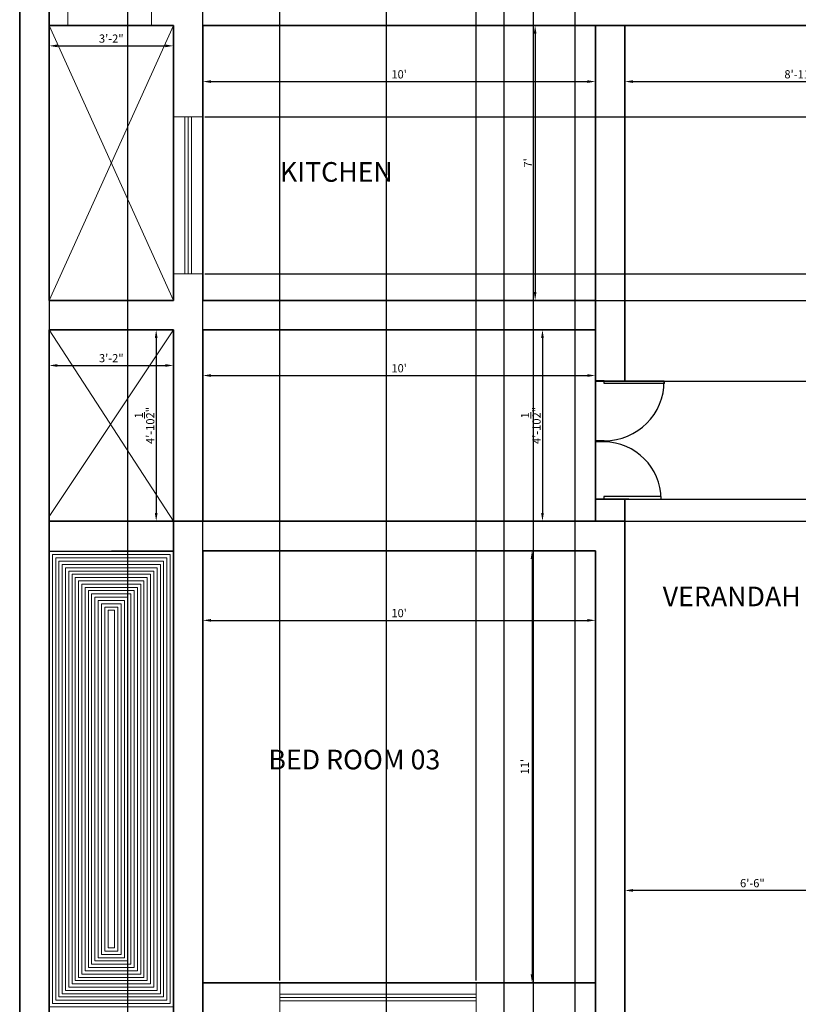
# Model space of a CAD drawing. Units: inches. Extents: x 2178 to 2667, y 1439 to 2239.
# Tile 2 of 5: x 2218 to 2456, y 1590 to 1891. Entities that reach past the tile are written whole.
import ezdxf

# ---------------------------------------------------------------- set-up
doc = ezdxf.new("R2010")
doc.units = ezdxf.units.IN
for name, color, linetype, lineweight in [('A-ANNO-DIMS', 2, 'Continuous', 18), ('A-AREA-IDEN', 7, 'Continuous', 18), ('A-DOOR', 3, 'Continuous', 25), ('A-FLOR-OPEN', 8, 'Continuous', 18), ('A-FLOR-PATT', 252, 'Continuous', 13), ('A-GLAZ', 4, 'Continuous', 18), ('A-WALL', 7, 'Continuous', 35)]:
    doc.layers.add(name, color=color, linetype=linetype, lineweight=lineweight)
doc.styles.get("Standard").update_dxf_attribs({"font": 'arial.ttf'})
doc.dimstyles.new('Copy of ISO-25', dxfattribs={"dimtxt": 2.5, "dimasz": 2.5, "dimexe": 1.25, "dimexo": 0.625, "dimtad": 1, "dimdec": 1, "dimlunit": 4, "dimtxsty": 'Standard', "dimcen": 2.5, "dimadec": 0, "dimazin": 0, "dimtfac": 1, "dimtdec": 1, "dimtmove": 0, "dimatfit": 3, "dimfxl": 1, "dimarcsym": 0})

# ---------------------------------------------------------------- blocks, each defined once
blk = doc.blocks.new('*D11')
at = {"layer": 'A-ANNO-DIMS', "color": 0, "lineweight": -2, "transparency": 16777216}
for p, q in [((2273.53, 1888.41), (2273.53, 1870.62)), ((2393.53, 1888.41), (2393.53, 1870.62)), ((2276.03, 1871.87), (2391.03, 1871.87))]:
    blk.add_line(p, q, dxfattribs=at)
at = {"layer": 'A-ANNO-DIMS', "color": 0, "transparency": 16777216}
for points in [[(2276.03, 1872.29), (2276.03, 1871.45), (2273.53, 1871.87)], [(2391.03, 1872.29), (2391.03, 1871.45), (2393.53, 1871.87)]]:
    blk.add_solid(points, dxfattribs=at)
at = {"layer": 'Defpoints', "color": 0, "transparency": 16777216}
for p in [(2273.53, 1889.03), (2393.53, 1889.03), (2393.53, 1871.87)]:
    blk.add_point(p, dxfattribs=at)
at = {"layer": 'A-ANNO-DIMS', "color": 0, "transparency": 16777216, "insert": (2333.53, 1873.77), "char_height": 2.5, "attachment_point": 5}
blk.add_mtext("10'", dxfattribs=at)
blk = doc.blocks.new('*D12')
at = {"layer": 'A-ANNO-DIMS', "color": 0, "lineweight": -2, "transparency": 16777216}
for p, q in [((2392.9, 1889.03), (2373.87, 1889.03)), ((2375.12, 1886.53), (2375.12, 1807.53)), ((2392.9, 1805.03), (2373.87, 1805.03))]:
    blk.add_line(p, q, dxfattribs=at)
at = {"layer": 'A-ANNO-DIMS', "color": 0, "transparency": 16777216}
for points in [[(2374.7, 1886.53), (2375.53, 1886.53), (2375.12, 1889.03)], [(2374.7, 1807.53), (2375.53, 1807.53), (2375.12, 1805.03)]]:
    blk.add_solid(points, dxfattribs=at)
at = {"layer": 'Defpoints', "color": 0, "transparency": 16777216}
for p in [(2393.53, 1889.03), (2375.12, 1805.03), (2393.53, 1805.03)]:
    blk.add_point(p, dxfattribs=at)
at = {"layer": 'A-ANNO-DIMS', "color": 0, "transparency": 16777216, "insert": (2373.24, 1847.03), "char_height": 2.5, "attachment_point": 5, "rotation": 90}
blk.add_mtext("7'", dxfattribs=at)
blk = doc.blocks.new('*D13')
at = {"layer": 'A-ANNO-DIMS', "color": 0, "lineweight": -2, "transparency": 16777216}
for p, q in [((2226.53, 1888.41), (2226.53, 1881.54)), ((2264.53, 1888.41), (2264.53, 1881.54)), ((2229.03, 1882.79), (2262.03, 1882.79))]:
    blk.add_line(p, q, dxfattribs=at)
at = {"layer": 'A-ANNO-DIMS', "color": 0, "transparency": 16777216}
for points in [[(2229.03, 1883.2), (2229.03, 1882.37), (2226.53, 1882.79)], [(2262.03, 1883.2), (2262.03, 1882.37), (2264.53, 1882.79)]]:
    blk.add_solid(points, dxfattribs=at)
at = {"layer": 'Defpoints', "color": 0, "transparency": 16777216}
for p in [(2226.53, 1889.03), (2264.53, 1889.03), (2264.53, 1882.79)]:
    blk.add_point(p, dxfattribs=at)
at = {"layer": 'A-ANNO-DIMS', "color": 0, "transparency": 16777216, "insert": (2245.53, 1884.69), "char_height": 2.5, "attachment_point": 5}
blk.add_mtext('3\'-2"', dxfattribs=at)
blk = doc.blocks.new('*D14')
at = {"layer": 'A-ANNO-DIMS', "color": 0, "lineweight": -2, "transparency": 16777216}
for p, q in [((2402.53, 1888.41), (2402.53, 1870.62)), ((2509.53, 1888.41), (2509.53, 1870.62)), ((2405.03, 1871.87), (2507.03, 1871.87))]:
    blk.add_line(p, q, dxfattribs=at)
at = {"layer": 'A-ANNO-DIMS', "color": 0, "transparency": 16777216}
for points in [[(2405.03, 1872.29), (2405.03, 1871.45), (2402.53, 1871.87)], [(2507.03, 1872.29), (2507.03, 1871.45), (2509.53, 1871.87)]]:
    blk.add_solid(points, dxfattribs=at)
at = {"layer": 'Defpoints', "color": 0, "transparency": 16777216}
for p in [(2402.53, 1889.03), (2509.53, 1889.03), (2509.53, 1871.87)]:
    blk.add_point(p, dxfattribs=at)
at = {"layer": 'A-ANNO-DIMS', "color": 0, "transparency": 16777216, "insert": (2456.03, 1873.77), "char_height": 2.5, "attachment_point": 5}
blk.add_mtext('8\'-11"', dxfattribs=at)
blk = doc.blocks.new('*D15')
at = {"layer": 'A-ANNO-DIMS', "color": 0, "lineweight": -2, "transparency": 16777216}
for p, q in [((2392.9, 1796.03), (2376.11, 1796.03)), ((2377.36, 1793.53), (2377.36, 1740.03)), ((2392.9, 1737.53), (2376.11, 1737.53))]:
    blk.add_line(p, q, dxfattribs=at)
at = {"layer": 'A-ANNO-DIMS', "color": 0, "transparency": 16777216}
for points in [[(2376.95, 1793.53), (2377.78, 1793.53), (2377.36, 1796.03)], [(2376.95, 1740.03), (2377.78, 1740.03), (2377.36, 1737.53)]]:
    blk.add_solid(points, dxfattribs=at)
at = {"layer": 'Defpoints', "color": 0, "transparency": 16777216}
for p in [(2393.53, 1796.03), (2377.36, 1737.53), (2393.53, 1737.53)]:
    blk.add_point(p, dxfattribs=at)
at = {"layer": 'A-ANNO-DIMS', "color": 0, "transparency": 16777216, "insert": (2373.79, 1766.78), "char_height": 2.5, "attachment_point": 5, "rotation": 90}
blk.add_mtext('4\'-10{\\H1x;\\S1/2;}"', dxfattribs=at)
blk = doc.blocks.new('*D16')
at = {"layer": 'A-ANNO-DIMS', "color": 0, "lineweight": -2, "transparency": 16777216}
for p, q in [((2226.53, 1795.41), (2226.53, 1783.88)), ((2264.53, 1795.41), (2264.53, 1783.88)), ((2229.03, 1785.13), (2262.03, 1785.13))]:
    blk.add_line(p, q, dxfattribs=at)
at = {"layer": 'A-ANNO-DIMS', "color": 0, "transparency": 16777216}
for points in [[(2229.03, 1785.54), (2229.03, 1784.71), (2226.53, 1785.13)], [(2262.03, 1785.54), (2262.03, 1784.71), (2264.53, 1785.13)]]:
    blk.add_solid(points, dxfattribs=at)
at = {"layer": 'Defpoints', "color": 0, "transparency": 16777216}
for p in [(2226.53, 1796.03), (2264.53, 1796.03), (2264.53, 1785.13)]:
    blk.add_point(p, dxfattribs=at)
at = {"layer": 'A-ANNO-DIMS', "color": 0, "transparency": 16777216, "insert": (2245.53, 1787.03), "char_height": 2.5, "attachment_point": 5}
blk.add_mtext('3\'-2"', dxfattribs=at)
blk = doc.blocks.new('*D17')
at = {"layer": 'A-ANNO-DIMS', "color": 0, "lineweight": -2, "transparency": 16777216}
for p, q in [((2263.9, 1796.03), (2258.01, 1796.03)), ((2259.26, 1793.53), (2259.26, 1740.03)), ((2263.9, 1737.53), (2258.01, 1737.53))]:
    blk.add_line(p, q, dxfattribs=at)
at = {"layer": 'A-ANNO-DIMS', "color": 0, "transparency": 16777216}
for points in [[(2258.85, 1793.53), (2259.68, 1793.53), (2259.26, 1796.03)], [(2258.85, 1740.03), (2259.68, 1740.03), (2259.26, 1737.53)]]:
    blk.add_solid(points, dxfattribs=at)
at = {"layer": 'Defpoints', "color": 0, "transparency": 16777216}
for p in [(2264.53, 1796.03), (2259.26, 1737.53), (2264.53, 1737.53)]:
    blk.add_point(p, dxfattribs=at)
at = {"layer": 'A-ANNO-DIMS', "color": 0, "transparency": 16777216, "insert": (2255.69, 1766.78), "char_height": 2.5, "attachment_point": 5, "rotation": 90}
blk.add_mtext('4\'-10{\\H1x;\\S1/2;}"', dxfattribs=at)
blk = doc.blocks.new('*D18')
at = {"layer": 'A-ANNO-DIMS', "color": 0, "lineweight": -2, "transparency": 16777216}
for p, q in [((2273.53, 1727.91), (2273.53, 1705.99)), ((2393.53, 1727.91), (2393.53, 1705.99)), ((2276.03, 1707.24), (2391.03, 1707.24))]:
    blk.add_line(p, q, dxfattribs=at)
at = {"layer": 'A-ANNO-DIMS', "color": 0, "transparency": 16777216}
for points in [[(2276.03, 1707.66), (2276.03, 1706.82), (2273.53, 1707.24)], [(2391.03, 1707.66), (2391.03, 1706.82), (2393.53, 1707.24)]]:
    blk.add_solid(points, dxfattribs=at)
at = {"layer": 'Defpoints', "color": 0, "transparency": 16777216}
for p in [(2273.53, 1728.53), (2393.53, 1728.53), (2393.53, 1707.24)]:
    blk.add_point(p, dxfattribs=at)
at = {"layer": 'A-ANNO-DIMS', "color": 0, "transparency": 16777216, "insert": (2333.53, 1709.14), "char_height": 2.5, "attachment_point": 5}
blk.add_mtext("10'", dxfattribs=at)
blk = doc.blocks.new('*D19')
at = {"layer": 'A-ANNO-DIMS', "color": 0, "lineweight": -2, "transparency": 16777216}
for p, q in [((2392.9, 1728.53), (2372.92, 1728.53)), ((2374.17, 1726.03), (2374.17, 1599.03)), ((2392.9, 1596.53), (2372.92, 1596.53))]:
    blk.add_line(p, q, dxfattribs=at)
at = {"layer": 'A-ANNO-DIMS', "color": 0, "transparency": 16777216}
for points in [[(2373.75, 1726.03), (2374.58, 1726.03), (2374.17, 1728.53)], [(2373.75, 1599.03), (2374.58, 1599.03), (2374.17, 1596.53)]]:
    blk.add_solid(points, dxfattribs=at)
at = {"layer": 'Defpoints', "color": 0, "transparency": 16777216}
for p in [(2393.53, 1728.53), (2374.17, 1596.53), (2393.53, 1596.53)]:
    blk.add_point(p, dxfattribs=at)
at = {"layer": 'A-ANNO-DIMS', "color": 0, "transparency": 16777216, "insert": (2372.29, 1662.53), "char_height": 2.5, "attachment_point": 5, "rotation": 90}
blk.add_mtext("11'", dxfattribs=at)
blk = doc.blocks.new('*D20')
at = {"layer": 'A-ANNO-DIMS', "color": 0, "lineweight": -2, "transparency": 16777216}
for p, q in [((2273.53, 1795.41), (2273.53, 1780.8)), ((2393.53, 1795.41), (2393.53, 1780.8)), ((2276.03, 1782.05), (2391.03, 1782.05))]:
    blk.add_line(p, q, dxfattribs=at)
at = {"layer": 'A-ANNO-DIMS', "color": 0, "transparency": 16777216}
for points in [[(2276.03, 1782.47), (2276.03, 1781.64), (2273.53, 1782.05)], [(2391.03, 1782.47), (2391.03, 1781.64), (2393.53, 1782.05)]]:
    blk.add_solid(points, dxfattribs=at)
at = {"layer": 'Defpoints', "color": 0, "transparency": 16777216}
for p in [(2273.53, 1796.03), (2393.53, 1796.03), (2393.53, 1782.05)]:
    blk.add_point(p, dxfattribs=at)
at = {"layer": 'A-ANNO-DIMS', "color": 0, "transparency": 16777216, "insert": (2333.53, 1783.95), "char_height": 2.5, "attachment_point": 5}
blk.add_mtext("10'", dxfattribs=at)
blk = doc.blocks.new('*D29')
at = {"layer": 'A-ANNO-DIMS', "color": 0, "lineweight": -2, "transparency": 16777216}
for p, q in [((2402.53, 1603.39), (2402.53, 1625.96)), ((2478.03, 1624.71), (2405.03, 1624.71)), ((2480.53, 1603.39), (2480.53, 1625.96))]:
    blk.add_line(p, q, dxfattribs=at)
at = {"layer": 'A-ANNO-DIMS', "color": 0, "transparency": 16777216}
for points in [[(2405.03, 1625.13), (2405.03, 1624.3), (2402.53, 1624.71)], [(2478.03, 1625.13), (2478.03, 1624.3), (2480.53, 1624.71)]]:
    blk.add_solid(points, dxfattribs=at)
at = {"layer": 'Defpoints', "color": 0, "transparency": 16777216}
for p in [(2402.53, 1624.71), (2402.53, 1602.76), (2480.53, 1602.76)]:
    blk.add_point(p, dxfattribs=at)
at = {"layer": 'A-ANNO-DIMS', "color": 0, "transparency": 16777216, "insert": (2441.53, 1626.61), "char_height": 2.5, "attachment_point": 5}
blk.add_mtext('6\'-6"', dxfattribs=at)
blk = doc.blocks.new('*U22')
for p, q in [((0, 0), (0, 6)), ((40, 0), (40, 6))]:
    blk.add_line(p, q)
blk.add_lwpolyline([(0, 0), (0, -40), (1.75, -40), (1.75, 0)], close=True)
blk.add_arc((0, 0), 40, 270, 0)
blk = doc.blocks.new('*U23')
for p, q in [((-40, 0), (-40, 6)), ((0, 0), (0, 6))]:
    blk.add_line(p, q)
blk.add_lwpolyline([(0, 0), (0, -40), (-1.75, -40), (-1.75, 0)], close=True)
blk.add_arc((0, 0), 40, 180, 270)
blk = doc.blocks.new('*D51')
at = {"layer": 'A-ANNO-DIMS', "color": 0, "lineweight": -2, "transparency": 16777216}
for p, q in [((2273.53, 1597.16), (2273.53, 2234.38)), ((2276.03, 2233.13), (2294.54, 2233.13)), ((2297.04, 1597.16), (2297.04, 2234.38))]:
    blk.add_line(p, q, dxfattribs=at)
at = {"layer": 'A-ANNO-DIMS', "color": 0, "transparency": 16777216}
for points in [[(2276.03, 2233.55), (2276.03, 2232.72), (2273.53, 2233.13)], [(2294.54, 2233.55), (2294.54, 2232.72), (2297.04, 2233.13)]]:
    blk.add_solid(points, dxfattribs=at)
at = {"layer": 'Defpoints', "color": 0, "transparency": 16777216}
for p in [(2297.04, 2233.13), (2273.53, 1596.53), (2297.04, 1596.53)]:
    blk.add_point(p, dxfattribs=at)
at = {"layer": 'A-ANNO-DIMS', "color": 0, "transparency": 16777216, "insert": (2285.28, 2235.05), "char_height": 2.5, "attachment_point": 5}
blk.add_mtext('1\'-11 1/2"', dxfattribs=at)
blk = doc.blocks.new('*D52')
at = {"layer": 'A-ANNO-DIMS', "color": 0, "lineweight": -2, "transparency": 16777216}
for p, q in [((2297.04, 1597.16), (2297.04, 2234.38)), ((2299.54, 2233.13), (2354.54, 2233.13)), ((2357.04, 1597.16), (2357.04, 2234.38))]:
    blk.add_line(p, q, dxfattribs=at)
at = {"layer": 'A-ANNO-DIMS', "color": 0, "transparency": 16777216}
for points in [[(2299.54, 2233.55), (2299.54, 2232.72), (2297.04, 2233.13)], [(2354.54, 2233.55), (2354.54, 2232.72), (2357.04, 2233.13)]]:
    blk.add_solid(points, dxfattribs=at)
at = {"layer": 'Defpoints', "color": 0, "transparency": 16777216}
for p in [(2357.04, 2233.13), (2297.04, 1596.53), (2357.04, 1596.53)]:
    blk.add_point(p, dxfattribs=at)
at = {"layer": 'A-ANNO-DIMS', "color": 0, "transparency": 16777216, "insert": (2327.04, 2235.04), "char_height": 2.5, "attachment_point": 5}
blk.add_mtext('5\'-0"', dxfattribs=at)
blk = doc.blocks.new('*D53')
at = {"layer": 'A-ANNO-DIMS', "color": 0, "lineweight": -2, "transparency": 16777216}
for p, q in [((2274.15, 1861.13), (2614.88, 1861.13)), ((2613.63, 1858.63), (2613.63, 1815.63)), ((2274.15, 1813.13), (2614.88, 1813.13))]:
    blk.add_line(p, q, dxfattribs=at)
at = {"layer": 'A-ANNO-DIMS', "color": 0, "transparency": 16777216}
for points in [[(2613.21, 1858.63), (2614.04, 1858.63), (2613.63, 1861.13)], [(2613.21, 1815.63), (2614.04, 1815.63), (2613.63, 1813.13)]]:
    blk.add_solid(points, dxfattribs=at)
at = {"layer": 'Defpoints', "color": 0, "transparency": 16777216}
for p in [(2273.53, 1861.13), (2273.53, 1813.13), (2613.63, 1813.13)]:
    blk.add_point(p, dxfattribs=at)
at = {"layer": 'A-ANNO-DIMS', "color": 0, "transparency": 16777216, "insert": (2611.72, 1837.13), "char_height": 2.5, "attachment_point": 5, "rotation": 90}
blk.add_mtext('4\'-0"', dxfattribs=at)
blk = doc.blocks.new('*D54')
at = {"layer": 'A-ANNO-DIMS', "color": 0, "lineweight": -2, "transparency": 16777216}
for p, q in [((2274.15, 1813.13), (2614.88, 1813.13)), ((2613.63, 1807.53), (2613.63, 1810.63)), ((2274.15, 1805.03), (2614.88, 1805.03))]:
    blk.add_line(p, q, dxfattribs=at)
at = {"layer": 'A-ANNO-DIMS', "color": 0, "transparency": 16777216}
for points in [[(2613.21, 1810.63), (2614.04, 1810.63), (2613.63, 1813.13)], [(2613.21, 1807.53), (2614.04, 1807.53), (2613.63, 1805.03)]]:
    blk.add_solid(points, dxfattribs=at)
at = {"layer": 'Defpoints', "color": 0, "transparency": 16777216}
for p in [(2273.53, 1813.13), (2613.63, 1813.13), (2273.53, 1805.03)]:
    blk.add_point(p, dxfattribs=at)
at = {"layer": 'A-ANNO-DIMS', "color": 0, "transparency": 16777216, "insert": (2611.72, 1809.08), "char_height": 2.5, "attachment_point": 5, "rotation": 90}
blk.add_mtext('0\'-8"', dxfattribs=at)
blk = doc.blocks.new('*D57')
at = {"layer": 'A-ANNO-DIMS', "color": 0, "lineweight": -2, "transparency": 16777216}
for p, q in [((2374.53, 2119.41), (2374.53, 1439.68)), ((2387.22, 2119.41), (2387.22, 1439.68)), ((2377.03, 1440.93), (2384.72, 1440.93)), ((2387.22, 1440.93), (2403.2, 1440.93))]:
    blk.add_line(p, q, dxfattribs=at)
at = {"layer": 'A-ANNO-DIMS', "color": 0, "transparency": 16777216}
for points in [[(2377.03, 1441.35), (2377.03, 1440.52), (2374.53, 1440.93)], [(2384.72, 1441.35), (2384.72, 1440.52), (2387.22, 1440.93)]]:
    blk.add_solid(points, dxfattribs=at)
at = {"layer": 'Defpoints', "color": 0, "transparency": 16777216}
for p in [(2374.53, 2120.03), (2387.22, 2120.03), (2387.22, 1440.93)]:
    blk.add_point(p, dxfattribs=at)
at = {"layer": 'A-ANNO-DIMS', "color": 0, "transparency": 16777216, "insert": (2396.46, 1442.85), "char_height": 2.5, "attachment_point": 5}
blk.add_mtext('1\'-0 1/2"', dxfattribs=at)
blk = doc.blocks.new('*D63')
at = {"layer": 'A-ANNO-DIMS', "color": 0, "lineweight": -2, "transparency": 16777216}
for p, q in [((2394.15, 1780.28), (2614.88, 1780.28)), ((2613.63, 1777.78), (2613.63, 1746.78)), ((2394.15, 1744.28), (2614.88, 1744.28))]:
    blk.add_line(p, q, dxfattribs=at)
at = {"layer": 'A-ANNO-DIMS', "color": 0, "transparency": 16777216}
for points in [[(2613.21, 1777.78), (2614.04, 1777.78), (2613.63, 1780.28)], [(2613.21, 1746.78), (2614.04, 1746.78), (2613.63, 1744.28)]]:
    blk.add_solid(points, dxfattribs=at)
at = {"layer": 'Defpoints', "color": 0, "transparency": 16777216}
for p in [(2393.53, 1780.28), (2393.53, 1744.28), (2613.63, 1744.28)]:
    blk.add_point(p, dxfattribs=at)
at = {"layer": 'A-ANNO-DIMS', "color": 0, "transparency": 16777216, "insert": (2611.72, 1762.28), "char_height": 2.5, "attachment_point": 5, "rotation": 90}
blk.add_mtext('3\'-0"', dxfattribs=at)
blk = doc.blocks.new('*D64')
at = {"layer": 'A-ANNO-DIMS', "color": 0, "lineweight": -2, "transparency": 16777216}
for p, q in [((2394.15, 1744.28), (2614.88, 1744.28)), ((2613.63, 1741.78), (2613.63, 1740.03)), ((2394.15, 1737.53), (2614.88, 1737.53)), ((2613.63, 1737.53), (2613.63, 1727.14))]:
    blk.add_line(p, q, dxfattribs=at)
at = {"layer": 'A-ANNO-DIMS', "color": 0, "transparency": 16777216}
for points in [[(2613.21, 1741.78), (2614.04, 1741.78), (2613.63, 1744.28)], [(2613.21, 1740.03), (2614.04, 1740.03), (2613.63, 1737.53)]]:
    blk.add_solid(points, dxfattribs=at)
at = {"layer": 'Defpoints', "color": 0, "transparency": 16777216}
for p in [(2393.53, 1744.28), (2393.53, 1737.53), (2613.63, 1737.53)]:
    blk.add_point(p, dxfattribs=at)
at = {"layer": 'A-ANNO-DIMS', "color": 0, "transparency": 16777216, "insert": (2611.72, 1731.09), "char_height": 2.5, "attachment_point": 5, "rotation": 90}
blk.add_mtext('0\'-7"', dxfattribs=at)
blk = doc.blocks.new('*D67')
at = {"layer": 'A-ANNO-DIMS', "color": 0, "lineweight": -2, "transparency": 16777216}
for p, q in [((2226.53, 2022.41), (2226.53, 1439.68)), ((2250.53, 2022.41), (2250.53, 1439.68)), ((2229.03, 1440.93), (2248.03, 1440.93))]:
    blk.add_line(p, q, dxfattribs=at)
at = {"layer": 'A-ANNO-DIMS', "color": 0, "transparency": 16777216}
for points in [[(2229.03, 1441.35), (2229.03, 1440.52), (2226.53, 1440.93)], [(2248.03, 1441.35), (2248.03, 1440.52), (2250.53, 1440.93)]]:
    blk.add_solid(points, dxfattribs=at)
at = {"layer": 'Defpoints', "color": 0, "transparency": 16777216}
for p in [(2226.53, 2023.03), (2250.53, 2023.03), (2250.53, 1440.93)]:
    blk.add_point(p, dxfattribs=at)
at = {"layer": 'A-ANNO-DIMS', "color": 0, "transparency": 16777216, "insert": (2238.53, 1442.84), "char_height": 2.5, "attachment_point": 5}
blk.add_mtext('2\'-0"', dxfattribs=at)
blk = doc.blocks.new('*D69')
at = {"layer": 'A-ANNO-DIMS', "color": 0, "lineweight": -2, "transparency": 16777216}
for p, q in [((2329.53, 2022.41), (2329.53, 1439.68)), ((2365.53, 2001.3), (2365.53, 1439.68)), ((2332.03, 1440.93), (2363.03, 1440.93))]:
    blk.add_line(p, q, dxfattribs=at)
at = {"layer": 'A-ANNO-DIMS', "color": 0, "transparency": 16777216}
for points in [[(2332.03, 1441.35), (2332.03, 1440.52), (2329.53, 1440.93)], [(2363.03, 1441.35), (2363.03, 1440.52), (2365.53, 1440.93)]]:
    blk.add_solid(points, dxfattribs=at)
at = {"layer": 'Defpoints', "color": 0, "transparency": 16777216}
for p in [(2329.53, 2023.03), (2365.53, 2001.92), (2365.53, 1440.93)]:
    blk.add_point(p, dxfattribs=at)
at = {"layer": 'A-ANNO-DIMS', "color": 0, "transparency": 16777216, "insert": (2347.53, 1442.84), "char_height": 2.5, "attachment_point": 5}
blk.add_mtext('3\'-0"', dxfattribs=at)

msp = doc.modelspace()

# ---------------------------------------------------------------- linework, layer by layer
at = {"layer": 'A-FLOR-OPEN'}
for p, q in [((2226.53, 1889.03), (2264.53, 1805.03)), ((2264.53, 1889.03), (2226.53, 1805.03)), ((2226.53, 1796.03), (2264.53, 1737.53)), ((2226.53, 1739), (2264.53, 1796.03)), ((2226.53, 1739), (2226.53, 1739))]:
    msp.add_line(p, q, dxfattribs=at)
at = {"layer": 'A-FLOR-PATT'}
for points in [[(2226.53, 1728.32), (2264.53, 1728.32), (2264.53, 1589.16), (2226.53, 1589.16)], [(2227.53, 1727.32), (2263.53, 1727.32), (2263.53, 1590.16), (2227.53, 1590.16)], [(2228.53, 1726.32), (2262.53, 1726.32), (2262.53, 1591.16), (2228.53, 1591.16)], [(2229.53, 1725.32), (2261.53, 1725.32), (2261.53, 1592.16), (2229.53, 1592.16)], [(2230.53, 1724.32), (2260.53, 1724.32), (2260.53, 1593.16), (2230.53, 1593.16)], [(2231.53, 1723.32), (2259.53, 1723.32), (2259.53, 1594.16), (2231.53, 1594.16)], [(2232.53, 1722.32), (2258.53, 1722.32), (2258.53, 1595.16), (2232.53, 1595.16)], [(2233.53, 1721.32), (2257.53, 1721.32), (2257.53, 1596.16), (2233.53, 1596.16)], [(2234.53, 1720.32), (2256.53, 1720.32), (2256.53, 1597.16), (2234.53, 1597.16)], [(2235.53, 1719.32), (2255.53, 1719.32), (2255.53, 1598.16), (2235.53, 1598.16)], [(2236.53, 1718.32), (2254.53, 1718.32), (2254.53, 1599.16), (2236.53, 1599.16)], [(2237.53, 1717.32), (2253.53, 1717.32), (2253.53, 1600.16), (2237.53, 1600.16)], [(2238.53, 1716.32), (2252.53, 1716.32), (2252.53, 1601.16), (2238.53, 1601.16)], [(2239.53, 1715.32), (2251.53, 1715.32), (2251.53, 1602.16), (2239.53, 1602.16)], [(2240.53, 1714.32), (2250.53, 1714.32), (2250.53, 1603.16), (2240.53, 1603.16)], [(2241.53, 1713.32), (2249.53, 1713.32), (2249.53, 1604.16), (2241.53, 1604.16)], [(2242.53, 1712.32), (2248.53, 1712.32), (2248.53, 1605.16), (2242.53, 1605.16)], [(2243.53, 1711.32), (2247.53, 1711.32), (2247.53, 1606.16), (2243.53, 1606.16)], [(2244.53, 1710.32), (2246.53, 1710.32), (2246.53, 1607.16), (2244.53, 1607.16)]]:
    msp.add_lwpolyline(points, close=True, dxfattribs=at)
at = {"layer": 'A-GLAZ'}
for p, q in [((2232.26, 1889.03), (2232.26, 1898.03)), ((2257.84, 1898.03), (2257.84, 1889.03)), ((2264.53, 1861.13), (2273.53, 1861.13)), ((2268.03, 1861.13), (2268.03, 1813.13)), ((2269.03, 1861.13), (2269.03, 1813.13)), ((2270.03, 1861.13), (2270.03, 1813.13)), ((2273.53, 1861.13), (2273.53, 1813.13)), ((2273.53, 1813.13), (2264.53, 1813.13)), ((2297.04, 1587.53), (2297.04, 1596.53)), ((2297.04, 1596.53), (2345.04, 1596.53)), ((2345.04, 1596.53), (2357.04, 1596.53)), ((2357.04, 1596.53), (2357.04, 1587.53)), ((2297.04, 1593.03), (2357.04, 1593.03)), ((2297.04, 1592.03), (2357.04, 1592.03)), ((2297.04, 1591.03), (2357.04, 1591.03))]:
    msp.add_line(p, q, dxfattribs=at)
at = {"layer": 'A-WALL'}
for p, q in [((2217.53, 1477.03), (2217.53, 2197.03)), ((2226.53, 1805.03), (2226.53, 2188.03)), ((2264.53, 1889.03), (2226.53, 1889.03)), ((2226.53, 1889.03), (2232.26, 1889.03)), ((2264.53, 1889.03), (2264.53, 1805.03)), ((2374.53, 1889.03), (2273.53, 1889.03)), ((2393.53, 1889.03), (2273.53, 1889.03)), ((2273.53, 1805.03), (2273.53, 1889.03)), ((2309.53, 1889.03), (2300.53, 1889.03)), ((2374.53, 1889.03), (2509.53, 1889.03)), ((2402.53, 1889.03), (2393.53, 1889.03)), ((2393.53, 1889.03), (2393.53, 1780.28)), ((2393.53, 1889.03), (2393.53, 1780.28)), ((2393.53, 1889.03), (2393.53, 1805.03)), ((2509.53, 1889.03), (2402.53, 1889.03)), ((2402.53, 1889.03), (2402.53, 1780.28)), ((2264.53, 1805.03), (2226.53, 1805.03)), ((2393.53, 1805.03), (2273.53, 1805.03)), ((2226.53, 1486.03), (2226.53, 1796.03)), ((2264.53, 1796.03), (2226.53, 1796.03)), ((2264.53, 1796.03), (2264.53, 1683.53)), ((2273.53, 1796.03), (2393.53, 1796.03)), ((2273.53, 1737.53), (2273.53, 1796.03)), ((2393.53, 1796.03), (2393.53, 1780.28)), ((2393.53, 1744.28), (2393.53, 1780.8)), ((2393.53, 1780.28), (2402.53, 1780.28)), ((2393.53, 1744.28), (2393.53, 1737.53)), ((2393.53, 1737.53), (2393.53, 1744.28)), ((2403.74, 1744.28), (2393.53, 1744.28)), ((2393.53, 1744.28), (2393.53, 1737.53)), ((2393.53, 1744.28), (2393.53, 1737.53)), ((2402.53, 1744.28), (2402.53, 1683.53)), ((2264.53, 1737.53), (2226.53, 1737.53)), ((2226.53, 1737.53), (2226.53, 1728.32)), ((2273.53, 1737.53), (2264.53, 1737.53)), ((2393.53, 1737.53), (2273.53, 1737.53)), ((2393.53, 1737.53), (2402.53, 1737.53)), ((2226.53, 1728.32), (2264.53, 1728.49)), ((2273.53, 1692.53), (2273.53, 1728.53)), ((2273.53, 1728.53), (2393.53, 1728.53)), ((2393.53, 1728.53), (2393.53, 1692.53)), ((2393.53, 1728.53), (2393.53, 1692.53)), ((2273.53, 1692.53), (2273.53, 1683.53)), ((2393.53, 1692.53), (2393.53, 1683.53)), ((2264.53, 1683.53), (2264.53, 1587.53)), ((2273.53, 1683.53), (2273.53, 1587.53)), ((2393.53, 1587.53), (2393.53, 1683.53)), ((2402.53, 1587.53), (2402.53, 1683.53)), ((2393.53, 1596.53), (2273.53, 1596.53)), ((2273.53, 1596.53), (2273.53, 1587.53)), ((2393.53, 1587.53), (2393.53, 1596.53))]:
    msp.add_line(p, q, dxfattribs=at)

# ---------------------------------------------------------------- block references
at = {"layer": 'A-DOOR', "rotation": 90}
for name, p, xscale, yscale, zscale in [('*U23', (2396.27, 1780.41), 0.4580787990422996, 0.4580787990422996, 0.4580787990422996), ('*U22', (2396.15, 1744.28), 0.4365934785165416, 0.4365934785165416, 0.4365934785165416)]:
    msp.add_blockref(name, p, dxfattribs=dict(at, xscale=xscale, yscale=yscale, zscale=zscale))

# ---------------------------------------------------------------- texts
at = {"layer": 'A-AREA-IDEN'}
for s, p in [('KITCHEN', (2297.09, 1841.27)), ('VERANDAH', (2414.12, 1711.55)), ('BED ROOM 03', (2293.55, 1661.71))]:
    msp.add_text(s, height=6, dxfattribs=at).set_placement(p)

# ---------------------------------------------------------------- dimensions: what is measured, and where the dimension line sits
at = {"layer": 'A-ANNO-DIMS'}
for base, p1, p2, override, picture, middle in [((2297.04, 2233.13), (2273.53, 1596.53), (2297.04, 1596.53), {"dimdec": 1, "dimlfac": 1, "dimrnd": 0, "dimzin": 1, "dimdsep": 46, "dimlunit": 4, "dimfrac": 2}, '*D51', (2285.28, 2235.05)), ((2357.04, 2233.13), (2297.04, 1596.53), (2357.04, 1596.53), {"dimdec": 1, "dimlfac": 1, "dimrnd": 0, "dimzin": 1, "dimdsep": 46, "dimlunit": 4, "dimfrac": 2}, '*D52', (2327.04, 2235.04)), ((2387.22, 1440.93), (2374.53, 2120.03), (2387.22, 2120.03), {"dimdec": 1, "dimlfac": 1, "dimrnd": 0, "dimzin": 1, "dimdsep": 46, "dimlunit": 4, "dimfrac": 2}, '*D57', (2396.46, 1442.85)), ((2250.53, 1440.93), (2226.53, 2023.03), (2250.53, 2023.03), {"dimdec": 1, "dimlfac": 1, "dimrnd": 0, "dimzin": 1, "dimdsep": 46, "dimlunit": 4, "dimfrac": 2}, '*D67', (2238.53, 1442.84)), ((2365.53, 1440.93), (2329.53, 2023.03), (2365.53, 2001.92), {"dimdec": 1, "dimlfac": 1, "dimrnd": 0, "dimzin": 1, "dimdsep": 46, "dimlunit": 4, "dimfrac": 2}, '*D69', (2347.53, 1442.84)), ((2264.53, 1882.79), (2226.53, 1889.03), (2264.53, 1889.03), {"dimclrd": 0, "dimclre": 0, "dimclrt": 0}, '*D13', (2245.53, 1884.69)), ((2393.53, 1871.87), (2273.53, 1889.03), (2393.53, 1889.03), {"dimclrd": 0, "dimclre": 0, "dimclrt": 0}, '*D11', (2333.53, 1873.77)), ((2509.53, 1871.87), (2402.53, 1889.03), (2509.53, 1889.03), {"dimclrd": 0, "dimclre": 0, "dimclrt": 0}, '*D14', (2456.03, 1873.77)), ((2264.53, 1785.13), (2226.53, 1796.03), (2264.53, 1796.03), {"dimclrd": 0, "dimclre": 0, "dimclrt": 0}, '*D16', (2245.53, 1787.03)), ((2393.53, 1782.05), (2273.53, 1796.03), (2393.53, 1796.03), {"dimclrd": 0, "dimclre": 0, "dimclrt": 0}, '*D20', (2333.53, 1783.95)), ((2393.53, 1707.24), (2273.53, 1728.53), (2393.53, 1728.53), {"dimclrd": 0, "dimclre": 0, "dimclrt": 0}, '*D18', (2333.53, 1709.14)), ((2402.53, 1624.71), (2480.53, 1602.76), (2402.53, 1602.76), {"dimclrd": 0, "dimclre": 0, "dimclrt": 0}, '*D29', (2441.53, 1626.61))]:
    dim = msp.add_linear_dim(base=base, p1=p1, p2=p2, dimstyle='Copy of ISO-25', override=override, dxfattribs=at)
    dim.commit()
    dim.dimension.update_dxf_attribs({"geometry": picture, "text_midpoint": middle})
for base, p1, p2, override, picture, middle in [((2375.12, 1805.03), (2393.53, 1889.03), (2393.53, 1805.03), {"dimclrd": 0, "dimclre": 0, "dimclrt": 0}, '*D12', (2373.24, 1847.03)), ((2613.63, 1813.13), (2273.53, 1861.13), (2273.53, 1813.13), {"dimdec": 1, "dimlfac": 1, "dimrnd": 0, "dimzin": 1, "dimdsep": 46, "dimlunit": 4, "dimfrac": 2}, '*D53', (2611.72, 1837.13)), ((2613.63, 1813.13), (2273.53, 1805.03), (2273.53, 1813.13), {"dimdec": 1, "dimlfac": 1, "dimrnd": 0, "dimzin": 1, "dimdsep": 46, "dimlunit": 4, "dimfrac": 2}, '*D54', (2611.72, 1809.08)), ((2259.26, 1737.53), (2264.53, 1796.03), (2264.53, 1737.53), {"dimclrd": 0, "dimclre": 0, "dimclrt": 0}, '*D17', (2255.69, 1766.78)), ((2377.36, 1737.53), (2393.53, 1796.03), (2393.53, 1737.53), {"dimclrd": 0, "dimclre": 0, "dimclrt": 0}, '*D15', (2373.79, 1766.78)), ((2613.63, 1744.28), (2393.53, 1780.28), (2393.53, 1744.28), {"dimdec": 1, "dimlfac": 1, "dimrnd": 0, "dimzin": 1, "dimdsep": 46, "dimlunit": 4, "dimfrac": 2}, '*D63', (2611.72, 1762.28)), ((2613.625586, 1737.534601), (2393.525586, 1744.284601), (2393.525586, 1737.534601), {"dimdec": 1, "dimlfac": 1, "dimrnd": 0, "dimzin": 1, "dimdsep": 46, "dimlunit": 4, "dimfrac": 2}, '*D64', (2611.72415353, 1731.08678381)), ((2374.17, 1596.53), (2393.53, 1728.53), (2393.53, 1596.53), {"dimclrd": 0, "dimclre": 0, "dimclrt": 0}, '*D19', (2372.29, 1662.53))]:
    dim = msp.add_linear_dim(base=base, p1=p1, p2=p2, angle=90, dimstyle='Copy of ISO-25', override=override, dxfattribs=at)
    dim.commit()
    dim.dimension.update_dxf_attribs({"geometry": picture, "text_midpoint": middle})

doc.saveas('drawing.dxf')
